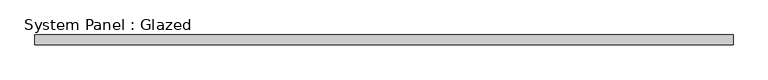
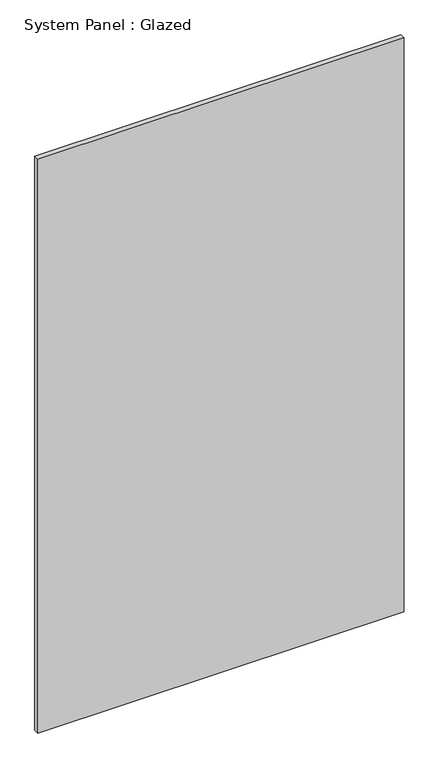
"""IFC4 building model written with IfcOpenShell, lengths in millimetres: plate geometry, System Panel : Glazed."""

from ifc_helpers import new_model, si_unit, origin, origin_with_axes, place, context, project, spatial, polyline, outline, extrude, source, transform, mapped, element, save


def system_panel_glazed_f5f8a0d0(model_context):
    return source(origin(), model_context, "Body", "SweptSolid", [
        extrude(outline(polyline([(905.9643899, 24.5), (-905.9643899, 24.5), (-905.9643899, 49.5), (905.9643899, 49.5), (905.9643899, 24.5)])), origin_with_axes(), (0.0, 0.0, 1.0), 3000.0),
    ])


if __name__ == "__main__":
    model = new_model("IFC4")
    model_context = context("Model", 3, world=origin())
    ifc_project = project(units=[si_unit("LENGTHUNIT", "METRE", prefix="MILLI")], contexts=[model_context])
    site = spatial("IfcSite", under=ifc_project)
    building = spatial("IfcBuilding", under=site)
    placement = place(None, origin())
    system_panel_glazed_shape = system_panel_glazed_f5f8a0d0(model_context)
    element("IfcPlate", 1, ObjectType="System Panel : Glazed", at=placement, inside=building, context=model_context, shape_type="MappedRepresentation", body=[
        mapped(system_panel_glazed_shape, transform((0.0, 0.0, 0.0), x_axis=(1.0, 0.0, 0.0), y_axis=(0.0, 1.0, 0.0), z_axis=(0.0, 0.0, 1.0))),
    ])
    save(model, "model.ifc")

# Revit data of these elements
# Type "System Panel : Glazed"
#   Keynote = "H11"
#   Construction Type Id = "GSP4R"
#   Analytic Construction = "1/8 in Pilkington single glazing"
#   Visual Light Transmittance = 0.9
#   Solar Heat Gain Coefficient = 0.86
#   Heat Transfer Coefficient (U) = 6.7069 W/(m²·K)
#   Define Thermal Properties by = 1
# Element 1 (IfcPlate, "System Panel : Glazed")
#   Materials on its faces: "Glass"
# Materials
#   "Glass": class "Glass", colour RGB 0 128 192, transparency 0.9, Description = "Soda Lime Glass", Cost = 0
